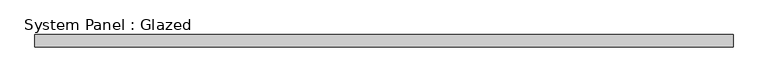
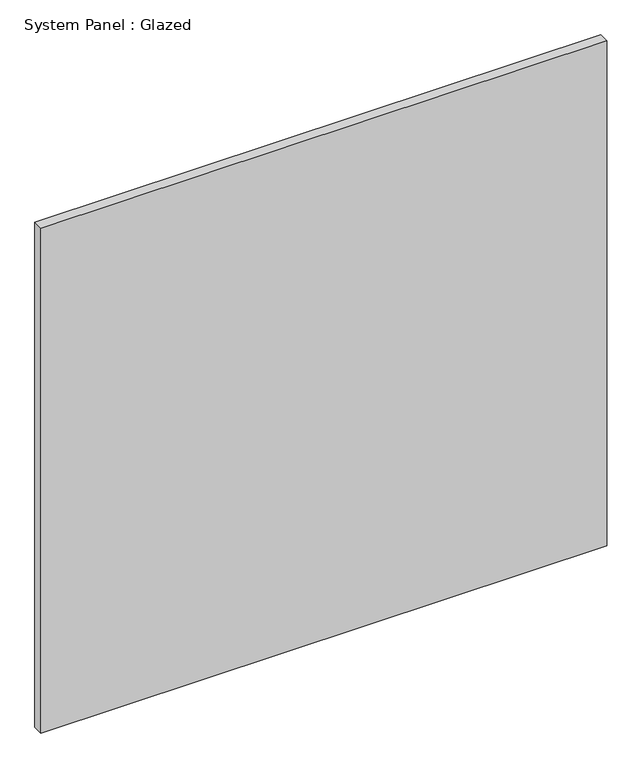
"""IFC4 building model written with IfcOpenShell, lengths in millimetres: plate geometry, System Panel : Glazed."""

from ifc_helpers import new_model, si_unit, origin, origin_with_axes, place, context, project, spatial, polyline, outline, extrude, source, transform, mapped, element, save


def system_panel_glazed_b6747f4f(model_context):
    return source(origin(), model_context, "Body", "SweptSolid", [
        extrude(outline(polyline([(705.589115, 24.5), (-705.589115, 24.5), (-705.589115, 49.5), (705.589115, 49.5), (705.589115, 24.5)])), origin_with_axes(), (0.0, 0.0, 1.0), 1330.8429687),
    ])


if __name__ == "__main__":
    model = new_model("IFC4")
    model_context = context("Model", 3, world=origin())
    ifc_project = project(units=[si_unit("LENGTHUNIT", "METRE", prefix="MILLI")], contexts=[model_context])
    site = spatial("IfcSite", under=ifc_project)
    building = spatial("IfcBuilding", under=site)
    placement = place(None, origin())
    system_panel_glazed_shape = system_panel_glazed_b6747f4f(model_context)
    element("IfcPlate", 1, ObjectType="System Panel : Glazed", at=placement, inside=building, context=model_context, shape_type="MappedRepresentation", body=[
        mapped(system_panel_glazed_shape, transform((0.0, 0.0, 0.0), x_axis=(1.0, 0.0, 0.0), y_axis=(0.0, 1.0, 0.0), z_axis=(0.0, 0.0, 1.0))),
    ])
    save(model, "model.ifc")

# Revit data of these elements
# Type "System Panel : Glazed"
#   Keynote = "H11"
#   Construction Type Id = "GSP4R"
#   Analytic Construction = "1/8 in Pilkington single glazing"
#   Visual Light Transmittance = 0.9
#   Solar Heat Gain Coefficient = 0.86
#   Heat Transfer Coefficient (U) = 6.7069 W/(m²·K)
#   Define Thermal Properties by = 1
# Element 1 (IfcPlate, "System Panel : Glazed")
#   Materials on its faces: "Glass"
# Materials
#   "Glass": class "Glass", colour RGB 0 128 192, transparency 0.9, Description = "Soda Lime Glass", Cost = 0
